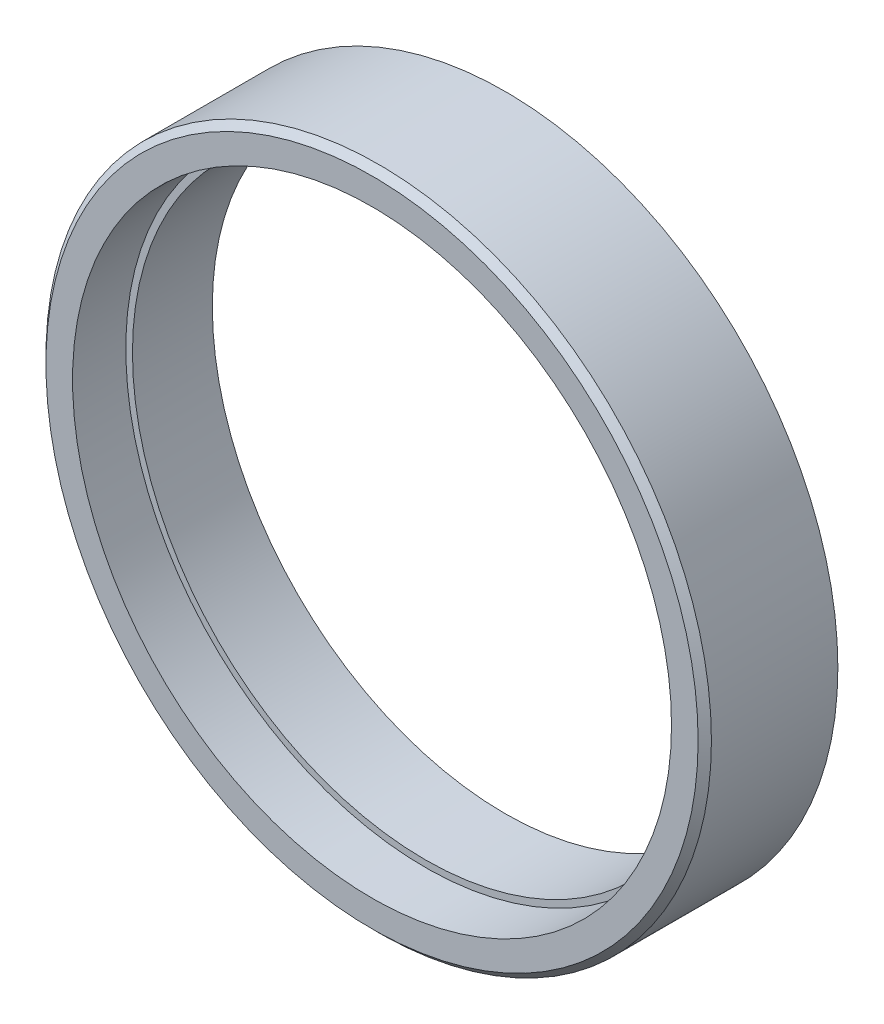
ISO-10303-21;
HEADER;
FILE_DESCRIPTION(('STEP AP214'),'2;1');
FILE_NAME('part.step','',(''),(''),'','','');
FILE_SCHEMA(('AUTOMOTIVE_DESIGN { 1 0 10303 214 1 1 1 1 }'));
ENDSEC;
DATA;
#1=APPLICATION_CONTEXT('core data for automotive mechanical design processes');
#2=APPLICATION_PROTOCOL_DEFINITION('international standard','automotive_design',2000,#1);
#3=PRODUCT_CONTEXT('',#1,'mechanical');
#4=PRODUCT('Part','Part','',(#3));
#5=PRODUCT_RELATED_PRODUCT_CATEGORY('part','',(#4));
#6=PRODUCT_DEFINITION_FORMATION('','',#4);
#7=PRODUCT_DEFINITION_CONTEXT('part definition',#1,'design');
#8=PRODUCT_DEFINITION('design','',#6,#7);
#9=PRODUCT_DEFINITION_SHAPE('','',#8);
#10=(LENGTH_UNIT() NAMED_UNIT(*) SI_UNIT(.MILLI.,.METRE.));
#11=(NAMED_UNIT(*) PLANE_ANGLE_UNIT() SI_UNIT($,.RADIAN.));
#12=(NAMED_UNIT(*) SI_UNIT($,.STERADIAN.) SOLID_ANGLE_UNIT());
#13=UNCERTAINTY_MEASURE_WITH_UNIT(LENGTH_MEASURE(1.E-05),#10,'distance_accuracy_value','');
#14=(GEOMETRIC_REPRESENTATION_CONTEXT(3) GLOBAL_UNCERTAINTY_ASSIGNED_CONTEXT((#13)) GLOBAL_UNIT_ASSIGNED_CONTEXT((#10,
#11,#12)) REPRESENTATION_CONTEXT('',''));
#15=CARTESIAN_POINT('',(0.,0.,0.));
#16=DIRECTION('',(0.,0.,1.));
#17=DIRECTION('',(1.,0.,0.));
#18=AXIS2_PLACEMENT_3D('',#15,#16,#17);
#19=CARTESIAN_POINT('',(0.,0.,20.));
#20=DIRECTION('',(0.,0.,-1.));
#21=DIRECTION('',(-1.,0.,0.));
#22=AXIS2_PLACEMENT_3D('',#19,#20,#21);
#23=CYLINDRICAL_SURFACE('',#22,50.);
#24=CARTESIAN_POINT('',(0.,0.,19.));
#25=DIRECTION('',(0.,0.,1.));
#26=DIRECTION('',(1.,0.,0.));
#27=AXIS2_PLACEMENT_3D('',#24,#25,#26);
#28=CIRCLE('',#27,50.);
#29=CARTESIAN_POINT('',(50.,0.,19.));
#30=VERTEX_POINT('',#29);
#31=EDGE_CURVE('E10',#30,#30,#28,.F.);
#32=ORIENTED_EDGE('',*,*,#31,.T.);
#33=EDGE_LOOP('',(#32));
#34=FACE_BOUND('',#33,.T.);
#35=CARTESIAN_POINT('',(0.,0.,0.));
#36=DIRECTION('',(0.,0.,1.));
#37=DIRECTION('',(1.,0.,0.));
#38=AXIS2_PLACEMENT_3D('',#35,#36,#37);
#39=CIRCLE('',#38,50.);
#40=CARTESIAN_POINT('',(50.,0.,0.));
#41=VERTEX_POINT('',#40);
#42=EDGE_CURVE('E51',#41,#41,#39,.T.);
#43=ORIENTED_EDGE('',*,*,#42,.T.);
#44=EDGE_LOOP('',(#43));
#45=FACE_BOUND('',#44,.T.);
#46=ADVANCED_FACE('F39',(#34,#45),#23,.T.);
#47=CARTESIAN_POINT('',(0.,0.,20.));
#48=DIRECTION('',(0.,0.,1.));
#49=DIRECTION('',(1.,0.,0.));
#50=AXIS2_PLACEMENT_3D('',#47,#48,#49);
#51=PLANE('',#50);
#52=CARTESIAN_POINT('',(0.,0.,20.));
#53=DIRECTION('',(0.,0.,1.));
#54=DIRECTION('',(1.,0.,0.));
#55=AXIS2_PLACEMENT_3D('',#52,#53,#54);
#56=CIRCLE('',#55,49.);
#57=CARTESIAN_POINT('',(49.,0.,20.));
#58=VERTEX_POINT('',#57);
#59=EDGE_CURVE('E50',#58,#58,#56,.T.);
#60=ORIENTED_EDGE('',*,*,#59,.T.);
#61=EDGE_LOOP('',(#60));
#62=FACE_BOUND('',#61,.T.);
#63=CARTESIAN_POINT('',(0.,0.,20.));
#64=DIRECTION('',(0.,0.,1.));
#65=DIRECTION('',(1.,0.,0.));
#66=AXIS2_PLACEMENT_3D('',#63,#64,#65);
#67=CIRCLE('',#66,45.);
#68=CARTESIAN_POINT('',(45.,0.,20.));
#69=VERTEX_POINT('',#68);
#70=EDGE_CURVE('E58',#69,#69,#67,.T.);
#71=ORIENTED_EDGE('',*,*,#70,.F.);
#72=EDGE_LOOP('',(#71));
#73=FACE_BOUND('',#72,.T.);
#74=ADVANCED_FACE('F88',(#62,#73),#51,.T.);
#75=CARTESIAN_POINT('',(0.,0.,0.));
#76=DIRECTION('',(0.,0.,1.));
#77=DIRECTION('',(1.,0.,0.));
#78=AXIS2_PLACEMENT_3D('',#75,#76,#77);
#79=PLANE('',#78);
#80=CARTESIAN_POINT('',(0.,0.,0.));
#81=DIRECTION('',(0.,0.,1.));
#82=DIRECTION('',(1.,0.,0.));
#83=AXIS2_PLACEMENT_3D('',#80,#81,#82);
#84=CIRCLE('',#83,44.);
#85=CARTESIAN_POINT('',(44.,0.,0.));
#86=VERTEX_POINT('',#85);
#87=EDGE_CURVE('E59',#86,#86,#84,.T.);
#88=ORIENTED_EDGE('',*,*,#87,.T.);
#89=EDGE_LOOP('',(#88));
#90=FACE_BOUND('',#89,.T.);
#91=ORIENTED_EDGE('',*,*,#42,.F.);
#92=EDGE_LOOP('',(#91));
#93=FACE_BOUND('',#92,.T.);
#94=ADVANCED_FACE('F82',(#90,#93),#79,.F.);
#95=CARTESIAN_POINT('',(0.,0.,12.));
#96=DIRECTION('',(0.,0.,1.));
#97=DIRECTION('',(1.,0.,0.));
#98=AXIS2_PLACEMENT_3D('',#95,#96,#97);
#99=CYLINDRICAL_SURFACE('',#98,45.);
#100=CARTESIAN_POINT('',(0.,0.,12.));
#101=DIRECTION('',(0.,0.,1.));
#102=DIRECTION('',(1.,0.,0.));
#103=AXIS2_PLACEMENT_3D('',#100,#101,#102);
#104=CIRCLE('',#103,45.);
#105=CARTESIAN_POINT('',(45.,0.,12.));
#106=VERTEX_POINT('',#105);
#107=EDGE_CURVE('E54',#106,#106,#104,.T.);
#108=ORIENTED_EDGE('',*,*,#107,.F.);
#109=EDGE_LOOP('',(#108));
#110=FACE_BOUND('',#109,.T.);
#111=ORIENTED_EDGE('',*,*,#70,.T.);
#112=EDGE_LOOP('',(#111));
#113=FACE_BOUND('',#112,.T.);
#114=ADVANCED_FACE('F78',(#110,#113),#99,.F.);
#115=CARTESIAN_POINT('',(0.,0.,12.));
#116=DIRECTION('',(0.,0.,1.));
#117=DIRECTION('',(1.,0.,0.));
#118=AXIS2_PLACEMENT_3D('',#115,#116,#117);
#119=PLANE('',#118);
#120=CARTESIAN_POINT('',(0.,0.,12.));
#121=DIRECTION('',(0.,0.,1.));
#122=DIRECTION('',(1.,0.,0.));
#123=AXIS2_PLACEMENT_3D('',#120,#121,#122);
#124=CIRCLE('',#123,44.);
#125=CARTESIAN_POINT('',(44.,0.,12.));
#126=VERTEX_POINT('',#125);
#127=EDGE_CURVE('E63',#126,#126,#124,.T.);
#128=ORIENTED_EDGE('',*,*,#127,.F.);
#129=EDGE_LOOP('',(#128));
#130=FACE_BOUND('',#129,.T.);
#131=ORIENTED_EDGE('',*,*,#107,.T.);
#132=EDGE_LOOP('',(#131));
#133=FACE_BOUND('',#132,.T.);
#134=ADVANCED_FACE('F71',(#130,#133),#119,.T.);
#135=CARTESIAN_POINT('',(0.,0.,-38.));
#136=DIRECTION('',(0.,0.,1.));
#137=DIRECTION('',(1.,0.,0.));
#138=AXIS2_PLACEMENT_3D('',#135,#136,#137);
#139=CYLINDRICAL_SURFACE('',#138,44.);
#140=ORIENTED_EDGE('',*,*,#127,.T.);
#141=EDGE_LOOP('',(#140));
#142=FACE_BOUND('',#141,.T.);
#143=ORIENTED_EDGE('',*,*,#87,.F.);
#144=EDGE_LOOP('',(#143));
#145=FACE_BOUND('',#144,.T.);
#146=ADVANCED_FACE('F70',(#142,#145),#139,.F.);
#147=CARTESIAN_POINT('',(0.,0.,20.));
#148=DIRECTION('',(0.,0.,-1.));
#149=DIRECTION('',(-1.,0.,0.));
#150=AXIS2_PLACEMENT_3D('',#147,#148,#149);
#151=CONICAL_SURFACE('',#150,49.,0.785398163397438);
#152=ORIENTED_EDGE('',*,*,#31,.F.);
#153=EDGE_LOOP('',(#152));
#154=FACE_BOUND('',#153,.T.);
#155=ORIENTED_EDGE('',*,*,#59,.F.);
#156=EDGE_LOOP('',(#155));
#157=FACE_BOUND('',#156,.T.);
#158=ADVANCED_FACE('F45',(#154,#157),#151,.T.);
#159=CLOSED_SHELL('',(#46,#74,#94,#114,#134,#146,#158));
#160=MANIFOLD_SOLID_BREP('B2',#159);
#161=ADVANCED_BREP_SHAPE_REPRESENTATION('',(#18,#160),#14);
#162=SHAPE_DEFINITION_REPRESENTATION(#9,#161);
ENDSEC;
END-ISO-10303-21;
